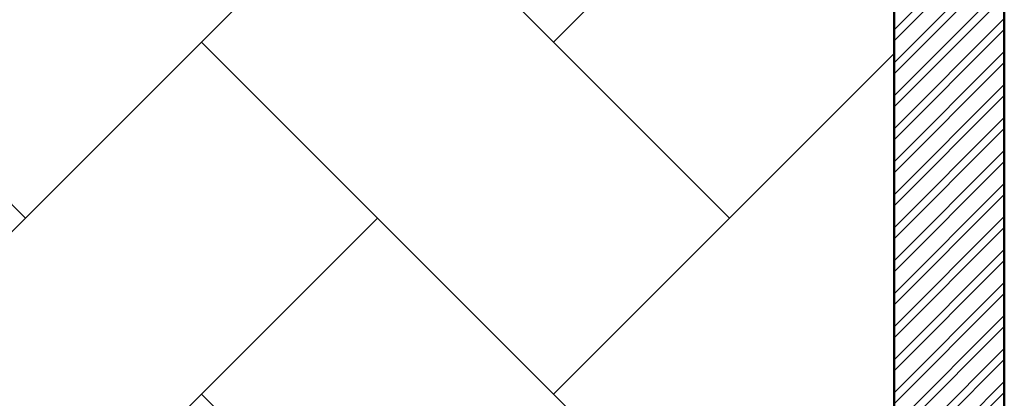
# Model space of a CAD drawing. Units: inches. Extents: x 3590 to 5167, y 65 to 1917.
# Tile 62 of 100: x 5000 to 5080, y 1609 to 1640. Entities that reach past the tile are written whole.
import ezdxf

# ---------------------------------------------------------------- set-up
doc = ezdxf.new("R2010")
doc.units = ezdxf.units.IN
for name, color, linetype, lineweight in [('A-FLOR-PATT', 8, 'Continuous', 13), ('A-WALL', 7, 'Continuous', 50), ('A-WALL-PATT', 251, 'Continuous', 13)]:
    doc.layers.add(name, color=color, linetype=linetype, lineweight=lineweight)

msp = doc.modelspace()

# ---------------------------------------------------------------- hatches: boundary and pattern name
at = {"layer": 'A-FLOR-PATT', "transparency": 33554687}
h = msp.add_hatch(dxfattribs=at)
h.set_pattern_fill('AR-HBONE', color=256, scale=0.2)
h.set_pattern_definition([(45, (-588.972, 0), (0, 28.73682), [60.96, -20.32]), (135, (-574.604, 14.368), (3e-15, 28.73682), [60.96, -20.32])])
h.paths.add_polyline_path([(5071.274, 1796.999), (4933.274, 1796.999), (4933.274, 1753.999), (4962.774, 1753.999, -0.414214), (4928.774, 1719.999), (4933.274, 1718.999), (4933.274, 1334.999), (5071.274, 1334.999)])
h.paths.add_polyline_path([(4951.78, 1521.077), (4951.715, 1521.04), (4951.563, 1520.895)], flags=16)
h.paths.add_polyline_path([(4952.267, 1521.376), (4952.198, 1521.371), (4952.198, 1521.356)], flags=0)
h.paths.add_polyline_path([(4967.051, 1529.728), (4965.231, 1528.694), (4963.411, 1527.714), (4961.756, 1526.851), (4963.589, 1527.449), (4964.036, 1527.478), (4962.975, 1527.249), (4961.76, 1526.852), (4959.792, 1525.834), (4958.005, 1524.895), (4956.24, 1523.93), (4954.504, 1522.919), (4954.129, 1522.682), (4953.361, 1521.997), (4953.366, 1521.998), (4953.605, 1522.064), (4955.106, 1522.761), (4956.921, 1523.434), (4958.678, 1523.915), (4960.358, 1524.2), (4961.945, 1524.286), (4964.171, 1524.108), (4965.958, 1523.309), (4963.863, 1522.976), (4965.187, 1522.499), (4963.366, 1522.497), (4961.545, 1522.487), (4959.764, 1522.461), (4958.304, 1522.419), (4957.974, 1522.388), (4956.307, 1522.232), (4954.718, 1522.071), (4953.251, 1521.899), (4953.525, 1521.623), (4954.331, 1521.379), (4956.243, 1521.23), (4958.039, 1520.93), (4959.684, 1520.483), (4961.16, 1519.896), (4963.107, 1518.8), (4964.393, 1517.325), (4962.973, 1517.726), (4964.558, 1516.661), (4965.407, 1515.708), (4963.507, 1516.322), (4961.68, 1517.005), (4959.935, 1517.745), (4958.282, 1518.528), (4956.732, 1519.343), (4955.295, 1520.175), (4954.672, 1520.572), (4954.513, 1520.627), (4955.658, 1519.318), (4956.703, 1517.982), (4957.644, 1516.647), (4958.485, 1515.334), (4959.55, 1513.524), (4960.438, 1511.769), (4958.841, 1513.62), (4957.452, 1515.325), (4955.819, 1517.459), (4956.665, 1515.448), (4957.111, 1513.923), (4957.447, 1511.714), (4957.076, 1509.793), (4956.538, 1511.11), (4955.992, 1512.569), (4955.444, 1514.125), (4954.898, 1515.735), (4954.357, 1517.356), (4953.824, 1518.943), (4953.305, 1520.452), (4953.065, 1521.116), (4952.971, 1521.146), (4952.949, 1521.086), (4952.73, 1520.199), (4953.37, 1518.024), (4953.757, 1516.373), (4954.051, 1514.765), (4954.264, 1513.221), (4954.471, 1511.131), (4954.497, 1510.402), (4954.409, 1511.76), (4954.264, 1513.221), (4954.051, 1514.765), (4953.757, 1516.373), (4953.37, 1518.024), (4952.877, 1519.698), (4952.716, 1520.141), (4952.533, 1519.059), (4952.374, 1517.789), (4952.219, 1516.312), (4952.046, 1514.6), (4951.833, 1512.626), (4951.557, 1510.363), (4951.203, 1512.168), (4950.852, 1514.339), (4950.985, 1516.376), (4951.66, 1518.286), (4952.593, 1520.481), (4952.357, 1521.13), (4951.855, 1520.328), (4950.839, 1518.908), (4949.777, 1517.587), (4948.916, 1516.617), (4948.111, 1515.256), (4947.089, 1513.554), (4945.889, 1511.615), (4946.326, 1513.402), (4946.562, 1514.249), (4945.528, 1513.327), (4944.581, 1512.531), (4946.018, 1514.508), (4947.204, 1516.048), (4947.893, 1517.313), (4949.307, 1518.764), (4950.414, 1519.767), (4950.451, 1519.806), (4952.267, 1521.376), (4951.645, 1521.493), (4950.404, 1521.18), (4948.044, 1520.359), (4946.119, 1519.452), (4944.572, 1518.475), (4943.35, 1517.443), (4941.997, 1515.92), (4941.661, 1515.275), (4942.813, 1516.99), (4944.572, 1518.475), (4946.119, 1519.452), (4948.044, 1520.359), (4950.404, 1521.18), (4951.645, 1521.493), (4949.647, 1521.868), (4948.6, 1521.756), (4947.126, 1521.57), (4945.42, 1521.348), (4943.45, 1521.105), (4941.183, 1520.856), (4942.86, 1521.613), (4943.873, 1522.03), (4942.952, 1521.909), (4941.41, 1521.485), (4939.543, 1520.67), (4938.968, 1520.226), (4940.733, 1521.299), (4942.952, 1521.909), (4943.702, 1522.008), (4945.894, 1522.7), (4947.565, 1522.714), (4948.921, 1522.566), (4951.131, 1522.183), (4950.971, 1522.297), (4948.129, 1523.006), (4946.035, 1523.707), (4944.232, 1524.521), (4942.707, 1525.461), (4941.444, 1526.537), (4940.43, 1527.761), (4939.649, 1529.143), (4941.421, 1528.122), (4943.147, 1527.132), (4944.841, 1526.175), (4946.514, 1525.25), (4948.179, 1524.359), (4948.365, 1524.263), (4946.475, 1526.045), (4945.181, 1527.54), (4944.19, 1529.033), (4943.496, 1530.54), (4943.278, 1531.36), (4942.498, 1531.919), (4943.114, 1531.762), (4942.959, 1533.659), (4944.14, 1531.989), (4944.612, 1531.323), (4946.202, 1530.463), (4947.486, 1529.509), (4948.79, 1528.226), (4950.368, 1526.237), (4949.485, 1528.155), (4948.851, 1530.123), (4948.491, 1532.041), (4948.381, 1533.918), (4948.501, 1535.76), (4948.827, 1537.573), (4949.418, 1535.565), (4949.957, 1533.569), (4950.464, 1531.586), (4950.961, 1529.617), (4951.391, 1527.954), (4951.724, 1530.687), (4952.201, 1532.58), (4952.889, 1534.33), (4953.77, 1535.951), (4954.827, 1537.46), (4954.521, 1535.39), (4954.273, 1533.937), (4955.58, 1535.663), (4956.748, 1536.739), (4956.159, 1534.78), (4955.589, 1532.873), (4955.043, 1531.006), (4954.525, 1529.166), (4954.038, 1527.341), (4953.638, 1525.733), (4953.611, 1525.586), (4953.398, 1524.166), (4953.382, 1524.009), (4954.07, 1525.476), (4954.912, 1527.022), (4956.136, 1528.894), (4957.847, 1530.577), (4959.376, 1531.54), (4958.256, 1530.104), (4957.143, 1528.663), (4956.066, 1527.243), (4955.056, 1525.871), (4954.141, 1524.571), (4953.352, 1523.372), (4953.311, 1523.303), (4953.273, 1522.925), (4953.261, 1522.382), (4954.103, 1523.373), (4954.63, 1524.284), (4955.961, 1526.358), (4957.23, 1528.13), (4958.421, 1529.609), (4960.037, 1531.368), (4961.374, 1532.375), (4962.101, 1532.77), (4961.07, 1531.061), (4959.987, 1529.438), (4958.869, 1527.908), (4958.15, 1527.007), (4959.803, 1528.003), (4961.589, 1528.793), (4963.391, 1529.328), (4965.211, 1529.632)], flags=16)
h.paths.add_polyline_path([(4962.944, 1523.182), (4961.107, 1523.422), (4960.392, 1523.362), (4962.35, 1523.331)], flags=0)
h.paths.add_polyline_path([(5049.541, 1584.551), (5049.476, 1584.515), (5049.325, 1584.37)], flags=16)
h.paths.add_polyline_path([(5050.028, 1584.851), (5049.959, 1584.845), (5049.959, 1584.83)], flags=0)
h.paths.add_polyline_path([(5042.333, 1581.949), (5043.88, 1582.926), (5045.806, 1583.833), (5048.165, 1584.654), (5049.406, 1584.967), (5047.408, 1585.342), (5046.361, 1585.231), (5044.888, 1585.044), (5043.181, 1584.822), (5041.211, 1584.579), (5038.944, 1584.33), (5040.622, 1585.087), (5041.634, 1585.504), (5040.713, 1585.383), (5039.171, 1584.959), (5037.304, 1584.144), (5036.729, 1583.7), (5038.494, 1584.773), (5040.713, 1585.383), (5041.463, 1585.482), (5043.655, 1586.174), (5045.326, 1586.188), (5046.682, 1586.04), (5048.893, 1585.657), (5048.732, 1585.771), (5045.891, 1586.48), (5043.796, 1587.181), (5041.994, 1587.996), (5040.468, 1588.935), (5039.205, 1590.011), (5038.191, 1591.235), (5037.41, 1592.617), (5039.182, 1591.596), (5040.909, 1590.607), (5042.602, 1589.649), (5044.275, 1588.724), (5045.94, 1587.833), (5046.126, 1587.738), (5044.237, 1589.519), (5042.942, 1591.015), (5041.952, 1592.508), (5041.257, 1594.014), (5041.039, 1594.834), (5040.26, 1595.393), (5040.875, 1595.237), (5040.721, 1597.133), (5041.901, 1595.463), (5042.373, 1594.798), (5043.963, 1593.938), (5045.247, 1592.983), (5046.552, 1591.701), (5048.129, 1589.712), (5047.247, 1591.63), (5046.613, 1593.597), (5046.252, 1595.515), (5046.142, 1597.392), (5046.262, 1599.234), (5046.588, 1601.047), (5047.179, 1599.039), (5047.718, 1597.043), (5048.225, 1595.06), (5048.722, 1593.091), (5049.152, 1591.429), (5049.485, 1594.161), (5049.962, 1596.054), (5050.65, 1597.804), (5051.532, 1599.425), (5052.589, 1600.934), (5052.283, 1598.864), (5052.034, 1597.411), (5053.341, 1599.137), (5054.509, 1600.213), (5053.92, 1598.254), (5053.35, 1596.348), (5052.805, 1594.48), (5052.286, 1592.64), (5051.799, 1590.815), (5051.4, 1589.207), (5051.373, 1589.06), (5051.159, 1587.64), (5051.143, 1587.483), (5051.831, 1588.95), (5052.673, 1590.496), (5053.898, 1592.368), (5055.608, 1594.051), (5057.137, 1595.014), (5056.017, 1593.578), (5054.904, 1592.137), (5053.828, 1590.717), (5052.817, 1589.345), (5051.902, 1588.046), (5051.113, 1586.846), (5051.072, 1586.777), (5051.034, 1586.399), (5051.022, 1585.856), (5051.864, 1586.847), (5052.391, 1587.758), (5053.723, 1589.832), (5054.991, 1591.604), (5056.182, 1593.083), (5057.798, 1594.842), (5059.135, 1595.849), (5059.863, 1596.244), (5058.831, 1594.535), (5057.749, 1592.912), (5056.63, 1591.382), (5055.912, 1590.482), (5057.564, 1591.477), (5059.35, 1592.267), (5061.152, 1592.802), (5062.972, 1593.106), (5064.812, 1593.203), (5062.992, 1592.169), (5061.172, 1591.188), (5059.518, 1590.325), (5061.35, 1590.924), (5061.797, 1590.952), (5060.737, 1590.723), (5059.521, 1590.326), (5057.553, 1589.308), (5055.766, 1588.369), (5054.002, 1587.404), (5052.265, 1586.393), (5051.891, 1586.156), (5051.122, 1585.471), (5051.127, 1585.472), (5051.366, 1585.538), (5052.867, 1586.235), (5054.682, 1586.908), (5056.439, 1587.389), (5058.12, 1587.675), (5059.706, 1587.76), (5061.933, 1587.583), (5063.719, 1586.783), (5061.624, 1586.45), (5062.949, 1585.973), (5061.127, 1585.971), (5059.307, 1585.961), (5057.525, 1585.935), (5056.065, 1585.893), (5055.735, 1585.862), (5054.068, 1585.707), (5052.479, 1585.546), (5051.012, 1585.373), (5051.286, 1585.097), (5052.092, 1584.853), (5054.004, 1584.704), (5055.8, 1584.404), (5057.446, 1583.958), (5058.921, 1583.37), (5060.868, 1582.274), (5062.154, 1580.799), (5060.734, 1581.2), (5062.32, 1580.135), (5063.168, 1579.182), (5061.269, 1579.796), (5059.441, 1580.479), (5057.696, 1581.219), (5056.043, 1582.003), (5054.493, 1582.817), (5053.057, 1583.649), (5052.433, 1584.047), (5052.274, 1584.101), (5053.42, 1582.793), (5054.464, 1581.457), (5055.405, 1580.121), (5056.247, 1578.809), (5057.311, 1576.998), (5058.199, 1575.244), (5056.602, 1577.094), (5055.213, 1578.799), (5053.58, 1580.933), (5054.427, 1578.922), (5054.872, 1577.397), (5055.208, 1575.189), (5054.838, 1573.267), (5054.299, 1574.584), (5053.754, 1576.043), (5053.206, 1577.599), (5052.659, 1579.209), (5052.118, 1580.83), (5051.585, 1582.417), (5051.066, 1583.927), (5050.826, 1584.59), (5050.733, 1584.62), (5050.711, 1584.561), (5050.491, 1583.673), (5051.131, 1581.498), (5051.518, 1579.847), (5051.813, 1578.24), (5052.026, 1576.695), (5052.233, 1574.605), (5052.258, 1573.876), (5052.17, 1575.234), (5052.026, 1576.695), (5051.813, 1578.24), (5051.518, 1579.847), (5051.131, 1581.498), (5050.638, 1583.172), (5050.477, 1583.615), (5050.294, 1582.533), (5050.136, 1581.263), (5049.981, 1579.786), (5049.807, 1578.074), (5049.594, 1576.1), (5049.318, 1573.837), (5048.965, 1575.642), (5048.613, 1577.813), (5048.747, 1579.85), (5049.421, 1581.76), (5050.354, 1583.955), (5050.118, 1584.604), (5049.616, 1583.802), (5048.6, 1582.382), (5047.538, 1581.061), (5046.677, 1580.091), (5045.872, 1578.73), (5044.85, 1577.028), (5043.651, 1575.089), (5044.087, 1576.877), (5044.324, 1577.723), (5043.289, 1576.801), (5042.342, 1576.005), (5043.779, 1577.982), (5044.966, 1579.522), (5045.655, 1580.787), (5047.068, 1582.239), (5048.175, 1583.241), (5048.213, 1583.28), (5050.028, 1584.851), (5049.406, 1584.967), (5048.165, 1584.654), (5045.806, 1583.833), (5043.88, 1582.926), (5042.333, 1581.949), (5041.111, 1580.917), (5039.758, 1579.394), (5039.423, 1578.749), (5040.575, 1580.464)], flags=16)
h.paths.add_polyline_path([(4954.799, 1533.12), (4954.262, 1532.079), (4953.831, 1530.935), (4953.505, 1529.636), (4953.283, 1528.133), (4953.167, 1526.376), (4953.156, 1524.315), (4953.277, 1521.236), (4952.802, 1521.842), (4951.557, 1521.998), (4950.976, 1521.961), (4952.661, 1521.941), (4952.802, 1521.842), (4953.152, 1523.593), (4953.167, 1526.376), (4953.283, 1528.133), (4953.609, 1530.346), (4954.456, 1532.592)], flags=0)
h.paths.add_polyline_path([(5050.563, 1585.316), (5049.318, 1585.472), (5048.737, 1585.435), (5050.422, 1585.415), (5050.563, 1585.316), (5050.914, 1587.067), (5050.928, 1589.851), (5051.045, 1591.607), (5051.371, 1593.82), (5052.217, 1596.066), (5052.56, 1596.594), (5052.024, 1595.554), (5051.592, 1594.409), (5051.266, 1593.11), (5051.045, 1591.607), (5050.928, 1589.851), (5050.918, 1587.789), (5051.038, 1584.71)], flags=0)
h.paths.add_polyline_path([(5058.153, 1586.836), (5060.111, 1586.805), (5060.705, 1586.656), (5058.868, 1586.896)], flags=0)
h.paths.add_polyline_path([(5049.541, 1430.936), (5049.476, 1430.9), (5049.325, 1430.755)], flags=16)
h.paths.add_polyline_path([(5050.028, 1431.236), (5049.959, 1431.231), (5049.959, 1431.215)], flags=0)
h.paths.add_polyline_path([(5046.588, 1447.432), (5047.179, 1445.425), (5047.718, 1443.429), (5048.225, 1441.446), (5048.722, 1439.476), (5049.152, 1437.814), (5049.485, 1440.546), (5049.962, 1442.439), (5050.65, 1444.189), (5051.532, 1445.811), (5052.589, 1447.319), (5052.283, 1445.249), (5052.034, 1443.796), (5053.341, 1445.522), (5054.509, 1446.598), (5053.92, 1444.64), (5053.35, 1442.733), (5052.805, 1440.865), (5052.286, 1439.025), (5051.799, 1437.201), (5051.4, 1435.592), (5051.373, 1435.445), (5051.159, 1434.025), (5051.143, 1433.868), (5051.831, 1435.335), (5052.673, 1436.881), (5053.898, 1438.753), (5055.608, 1440.436), (5057.137, 1441.4), (5056.017, 1439.963), (5054.904, 1438.522), (5053.828, 1437.102), (5052.817, 1435.73), (5051.902, 1434.431), (5051.113, 1433.231), (5051.072, 1433.162), (5051.034, 1432.784), (5051.022, 1432.242), (5051.864, 1433.232), (5052.391, 1434.143), (5053.723, 1436.217), (5054.991, 1437.989), (5056.182, 1439.468), (5057.798, 1441.227), (5059.135, 1442.235), (5059.863, 1442.629), (5058.831, 1440.921), (5057.749, 1439.298), (5056.63, 1437.767), (5055.912, 1436.867), (5057.564, 1437.863), (5059.35, 1438.652), (5061.152, 1439.187), (5062.972, 1439.491), (5064.812, 1439.588), (5062.992, 1438.554), (5061.172, 1437.573), (5059.518, 1436.71), (5061.35, 1437.309), (5061.797, 1437.337), (5060.737, 1437.108), (5059.521, 1436.711), (5057.553, 1435.693), (5055.766, 1434.754), (5054.002, 1433.789), (5052.265, 1432.778), (5051.891, 1432.541), (5051.122, 1431.856), (5051.127, 1431.857), (5051.366, 1431.923), (5052.867, 1432.62), (5054.682, 1433.293), (5056.439, 1433.775), (5058.12, 1434.06), (5059.706, 1434.145), (5061.933, 1433.968), (5063.719, 1433.168), (5061.624, 1432.835), (5062.949, 1432.358), (5061.127, 1432.357), (5059.307, 1432.346), (5057.525, 1432.32), (5056.065, 1432.278), (5055.735, 1432.248), (5054.068, 1432.092), (5052.479, 1431.931), (5051.012, 1431.759), (5051.286, 1431.482), (5052.092, 1431.238), (5054.004, 1431.089), (5055.8, 1430.789), (5057.446, 1430.343), (5058.921, 1429.755), (5060.868, 1428.66), (5062.154, 1427.185), (5060.734, 1427.585), (5062.32, 1426.52), (5063.168, 1425.567), (5061.269, 1426.181), (5059.441, 1426.865), (5057.696, 1427.604), (5056.043, 1428.388), (5054.493, 1429.202), (5053.057, 1430.034), (5052.433, 1430.432), (5052.274, 1430.487), (5053.42, 1429.178), (5054.464, 1427.842), (5055.405, 1426.506), (5056.247, 1425.194), (5057.311, 1423.383), (5058.199, 1421.629), (5056.602, 1423.479), (5055.213, 1425.184), (5053.58, 1427.318), (5054.427, 1425.307), (5054.872, 1423.782), (5055.208, 1421.574), (5054.838, 1419.652), (5054.299, 1420.97), (5053.754, 1422.428), (5053.206, 1423.984), (5052.659, 1425.595), (5052.118, 1427.215), (5051.585, 1428.802), (5051.066, 1430.312), (5050.826, 1430.975), (5050.733, 1431.005), (5050.711, 1430.946), (5050.491, 1430.058), (5051.131, 1427.883), (5051.518, 1426.232), (5051.813, 1424.625), (5052.026, 1423.081), (5052.233, 1420.991), (5052.258, 1420.261), (5052.17, 1421.619), (5052.026, 1423.081), (5051.813, 1424.625), (5051.518, 1426.232), (5051.131, 1427.883), (5050.638, 1429.558), (5050.477, 1430.001), (5050.294, 1428.918), (5050.136, 1427.648), (5049.981, 1426.171), (5049.807, 1424.459), (5049.594, 1422.485), (5049.318, 1420.222), (5048.965, 1422.028), (5048.613, 1424.199), (5048.747, 1426.235), (5049.421, 1428.146), (5050.354, 1430.34), (5050.118, 1430.989), (5049.616, 1430.187), (5048.6, 1428.768), (5047.538, 1427.446), (5046.677, 1426.477), (5045.872, 1425.116), (5044.85, 1423.413), (5043.651, 1421.474), (5044.087, 1423.262), (5044.324, 1424.109), (5043.289, 1423.186), (5042.342, 1422.391), (5043.779, 1424.368), (5044.966, 1425.907), (5045.655, 1427.173), (5047.068, 1428.624), (5048.175, 1429.627), (5048.213, 1429.666), (5050.028, 1431.236), (5049.406, 1431.353), (5048.165, 1431.039), (5045.806, 1430.218), (5043.88, 1429.311), (5042.333, 1428.334), (5041.111, 1427.302), (5039.758, 1425.779), (5039.423, 1425.134), (5040.575, 1426.849), (5042.333, 1428.334), (5043.88, 1429.311), (5045.806, 1430.218), (5048.165, 1431.039), (5049.406, 1431.353), (5047.408, 1431.727), (5046.361, 1431.616), (5044.888, 1431.429), (5043.181, 1431.207), (5041.211, 1430.964), (5038.944, 1430.715), (5040.622, 1431.472), (5041.634, 1431.89), (5040.713, 1431.769), (5039.171, 1431.345), (5037.304, 1430.53), (5036.729, 1430.085), (5038.494, 1431.158), (5040.713, 1431.769), (5041.463, 1431.867), (5043.655, 1432.559), (5045.326, 1432.573), (5046.682, 1432.425), (5048.893, 1432.042), (5048.732, 1432.156), (5045.891, 1432.865), (5043.796, 1433.566), (5041.994, 1434.381), (5040.468, 1435.321), (5039.205, 1436.396), (5038.191, 1437.62), (5037.41, 1439.002), (5039.182, 1437.982), (5040.909, 1436.992), (5042.602, 1436.034), (5044.275, 1435.109), (5045.94, 1434.218), (5046.126, 1434.123), (5044.237, 1435.904), (5042.942, 1437.4), (5041.952, 1438.893), (5041.257, 1440.399), (5041.039, 1441.219), (5040.26, 1441.778), (5040.875, 1441.622), (5040.721, 1443.518), (5041.901, 1441.848), (5042.373, 1441.183), (5043.963, 1440.323), (5045.247, 1439.369), (5046.552, 1438.086), (5048.129, 1436.097), (5047.247, 1438.015), (5046.613, 1439.982), (5046.252, 1441.901), (5046.142, 1443.778), (5046.262, 1445.619)], flags=16)
h.paths.add_polyline_path([(5052.382, 1444.255), (5051.623, 1442.78), (5052.024, 1441.939), (5052.56, 1442.98)], flags=0)
h.paths.add_polyline_path([(5050.563, 1431.701), (5049.318, 1431.857), (5048.737, 1431.821), (5050.422, 1431.8)], flags=0)
h.paths.add_polyline_path([(5058.153, 1433.221), (5060.111, 1433.19), (5060.705, 1433.041), (5058.868, 1433.281)], flags=0)
h.paths.add_polyline_path([(5049.541, 1352.285), (5049.476, 1352.249), (5049.325, 1352.104)], flags=16)
h.paths.add_polyline_path([(5050.028, 1352.585), (5049.959, 1352.58), (5049.959, 1352.564)], flags=0)
h.paths.add_polyline_path([(5046.588, 1368.781), (5047.179, 1366.774), (5047.718, 1364.778), (5048.225, 1362.795), (5048.722, 1360.825), (5049.152, 1359.163), (5049.485, 1361.896), (5049.962, 1363.789), (5050.65, 1365.538), (5051.532, 1367.16), (5052.589, 1368.669), (5052.283, 1366.598), (5052.034, 1365.145), (5053.341, 1366.871), (5054.509, 1367.947), (5053.92, 1365.989), (5053.35, 1364.082), (5052.805, 1362.214), (5052.286, 1360.374), (5051.799, 1358.55), (5051.4, 1356.942), (5051.373, 1356.794), (5051.159, 1355.374), (5051.143, 1355.218), (5051.831, 1356.684), (5052.673, 1358.23), (5053.898, 1360.102), (5055.608, 1361.786), (5057.137, 1362.749), (5056.017, 1361.313), (5054.904, 1359.872), (5053.828, 1358.452), (5052.817, 1357.079), (5051.902, 1355.78), (5051.113, 1354.581), (5051.072, 1354.512), (5051.034, 1354.133), (5051.022, 1353.591), (5051.864, 1354.581), (5052.391, 1355.492), (5053.723, 1357.566), (5054.991, 1359.338), (5056.182, 1360.817), (5057.798, 1362.577), (5059.135, 1363.584), (5059.863, 1363.979), (5058.831, 1362.27), (5057.749, 1360.647), (5056.63, 1359.117), (5055.912, 1358.216), (5057.564, 1359.212), (5059.35, 1360.001), (5061.152, 1360.536), (5062.972, 1360.841), (5064.812, 1360.937), (5062.992, 1359.903), (5061.172, 1358.923), (5059.518, 1358.059), (5061.35, 1358.658), (5061.797, 1358.687), (5060.737, 1358.458), (5059.521, 1358.061), (5057.553, 1357.043), (5055.766, 1356.103), (5054.002, 1355.138), (5052.265, 1354.127), (5051.891, 1353.89), (5051.122, 1353.206), (5051.127, 1353.206), (5051.366, 1353.272), (5052.867, 1353.969), (5054.682, 1354.643), (5056.439, 1355.124), (5058.12, 1355.409), (5059.706, 1355.495), (5061.933, 1355.317), (5063.719, 1354.518), (5061.624, 1354.184), (5062.949, 1353.708), (5061.127, 1353.706), (5059.307, 1353.695), (5057.525, 1353.669), (5056.065, 1353.627), (5055.735, 1353.597), (5054.068, 1353.441), (5052.479, 1353.28), (5051.012, 1353.108), (5051.286, 1352.831), (5052.092, 1352.587), (5054.004, 1352.439), (5055.8, 1352.138), (5057.446, 1351.692), (5058.921, 1351.104), (5060.868, 1350.009), (5062.154, 1348.534), (5060.734, 1348.935), (5062.32, 1347.869), (5063.168, 1346.916), (5061.269, 1347.53), (5059.441, 1348.214), (5057.696, 1348.954), (5056.043, 1349.737), (5054.493, 1350.551), (5053.057, 1351.383), (5052.433, 1351.781), (5052.274, 1351.836), (5053.42, 1350.527), (5054.464, 1349.191), (5055.405, 1347.855), (5056.247, 1346.543), (5057.311, 1344.733), (5058.199, 1342.978), (5056.602, 1344.828), (5055.213, 1346.534), (5053.58, 1348.667), (5054.427, 1346.656), (5054.872, 1345.132), (5055.208, 1342.923), (5054.838, 1341.002), (5054.299, 1342.319), (5053.754, 1343.778), (5053.206, 1345.334), (5052.659, 1346.944), (5052.118, 1348.564), (5051.585, 1350.151), (5051.066, 1351.661), (5050.826, 1352.324), (5050.733, 1352.355), (5050.711, 1352.295), (5050.491, 1351.408), (5051.131, 1349.232), (5051.518, 1347.581), (5051.813, 1345.974), (5052.026, 1344.43), (5052.233, 1342.34), (5052.258, 1341.61), (5052.17, 1342.969), (5052.026, 1344.43), (5051.813, 1345.974), (5051.518, 1347.581), (5051.131, 1349.232), (5050.638, 1350.907), (5050.477, 1351.35), (5050.294, 1350.267), (5050.136, 1348.997), (5049.981, 1347.52), (5049.807, 1345.809), (5049.594, 1343.835), (5049.318, 1341.571), (5048.965, 1343.377), (5048.613, 1345.548), (5048.747, 1347.585), (5049.421, 1349.495), (5050.354, 1351.689), (5050.118, 1352.339), (5049.616, 1351.536), (5048.6, 1350.117), (5047.538, 1348.795), (5046.677, 1347.826), (5045.872, 1346.465), (5044.85, 1344.763), (5043.651, 1342.824), (5044.087, 1344.611), (5044.324, 1345.458), (5043.289, 1344.535), (5042.342, 1343.74), (5043.779, 1345.717), (5044.966, 1347.256), (5045.655, 1348.522), (5047.068, 1349.973), (5048.175, 1350.976), (5048.213, 1351.015), (5050.028, 1352.585), (5049.406, 1352.702), (5048.165, 1352.388), (5045.806, 1351.567), (5043.88, 1350.661), (5042.333, 1349.683), (5041.111, 1348.651), (5039.758, 1347.128), (5039.423, 1346.483), (5040.575, 1348.198), (5042.333, 1349.683), (5043.88, 1350.661), (5045.806, 1351.567), (5048.165, 1352.388), (5049.406, 1352.702), (5047.408, 1353.076), (5046.361, 1352.965), (5044.888, 1352.779), (5043.181, 1352.556), (5041.211, 1352.313), (5038.944, 1352.065), (5040.622, 1352.821), (5041.634, 1353.239), (5040.713, 1353.118), (5039.171, 1352.694), (5037.304, 1351.879), (5036.729, 1351.434), (5038.494, 1352.508), (5040.713, 1353.118), (5041.463, 1353.216), (5043.655, 1353.909), (5045.326, 1353.923), (5046.682, 1353.774), (5048.893, 1353.391), (5048.732, 1353.506), (5045.891, 1354.214), (5043.796, 1354.915), (5041.994, 1355.73), (5040.468, 1356.67), (5039.205, 1357.746), (5038.191, 1358.969), (5037.41, 1360.352), (5039.182, 1359.331), (5040.909, 1358.341), (5042.602, 1357.383), (5044.275, 1356.458), (5045.94, 1355.567), (5046.126, 1355.472), (5044.237, 1357.253), (5042.942, 1358.749), (5041.952, 1360.242), (5041.257, 1361.748), (5041.039, 1362.568), (5040.26, 1363.128), (5040.875, 1362.971), (5040.721, 1364.867), (5041.901, 1363.197), (5042.373, 1362.532), (5043.963, 1361.672), (5045.247, 1360.718), (5046.552, 1359.435), (5048.129, 1357.446), (5047.247, 1359.364), (5046.613, 1361.331), (5046.252, 1363.25), (5046.142, 1365.127), (5046.262, 1366.969)], flags=16)
h.paths.add_polyline_path([(5052.382, 1365.604), (5051.623, 1364.129), (5052.024, 1363.288), (5052.56, 1364.329)], flags=0)
h.paths.add_polyline_path([(4951.78, 1698.041), (4951.715, 1698.005), (4951.563, 1697.859)], flags=16)
h.paths.add_polyline_path([(4952.267, 1698.341), (4952.198, 1698.335), (4952.198, 1698.32)], flags=0)
h.paths.add_polyline_path([(4957.076, 1686.757), (4956.538, 1688.074), (4955.992, 1689.533), (4955.444, 1691.089), (4954.898, 1692.699), (4954.357, 1694.32), (4953.824, 1695.907), (4953.305, 1697.417), (4953.065, 1698.08), (4952.971, 1698.11), (4952.949, 1698.051), (4952.73, 1697.163), (4953.37, 1694.988), (4953.757, 1693.337), (4954.051, 1691.729), (4954.264, 1690.185), (4954.471, 1688.095), (4954.497, 1687.366), (4954.409, 1688.724), (4954.264, 1690.185), (4954.051, 1691.729), (4953.757, 1693.337), (4953.37, 1694.988), (4952.877, 1696.662), (4952.716, 1697.105), (4952.533, 1696.023), (4952.374, 1694.753), (4952.219, 1693.276), (4952.046, 1691.564), (4951.833, 1689.59), (4951.557, 1687.327), (4951.203, 1689.132), (4950.852, 1691.303), (4950.985, 1693.34), (4951.66, 1695.25), (4952.593, 1697.445), (4952.357, 1698.094), (4951.855, 1697.292), (4950.839, 1695.872), (4949.777, 1694.551), (4948.916, 1693.581), (4948.111, 1692.22), (4947.089, 1690.518), (4945.889, 1688.579), (4946.326, 1690.366), (4946.562, 1691.213), (4945.528, 1690.291), (4944.581, 1689.495), (4946.018, 1691.472), (4947.204, 1693.012), (4947.893, 1694.277), (4949.307, 1695.729), (4950.414, 1696.731), (4950.451, 1696.77), (4952.267, 1698.341), (4951.645, 1698.457), (4950.404, 1698.144), (4948.044, 1697.323), (4946.119, 1696.416), (4944.572, 1695.439), (4943.35, 1694.407), (4941.997, 1692.884), (4941.661, 1692.239), (4942.813, 1693.954), (4944.572, 1695.439), (4946.119, 1696.416), (4948.044, 1697.323), (4950.404, 1698.144), (4951.645, 1698.457), (4949.647, 1698.832), (4948.6, 1698.72), (4947.126, 1698.534), (4945.42, 1698.312), (4943.45, 1698.069), (4941.183, 1697.82), (4942.86, 1698.577), (4943.873, 1698.994), (4942.952, 1698.873), (4941.41, 1698.449), (4939.543, 1697.634), (4938.968, 1697.19), (4940.733, 1698.263), (4942.952, 1698.873), (4943.702, 1698.972), (4945.894, 1699.664), (4947.565, 1699.678), (4948.921, 1699.53), (4951.131, 1699.147), (4950.971, 1699.261), (4948.129, 1699.97), (4946.035, 1700.671), (4944.232, 1701.486), (4942.707, 1702.425), (4941.444, 1703.501), (4940.43, 1704.725), (4939.649, 1706.107), (4941.421, 1705.086), (4943.147, 1704.097), (4944.841, 1703.139), (4946.514, 1702.214), (4948.179, 1701.323), (4948.365, 1701.227), (4946.475, 1703.009), (4945.181, 1704.505), (4944.19, 1705.997), (4943.496, 1707.504), (4943.278, 1708.324), (4942.498, 1708.883), (4943.114, 1708.727), (4942.959, 1710.623), (4944.14, 1708.953), (4944.612, 1708.287), (4946.202, 1707.428), (4947.486, 1706.473), (4948.79, 1705.191), (4950.368, 1703.202), (4949.485, 1705.12), (4948.851, 1707.087), (4948.491, 1709.005), (4948.381, 1710.882), (4948.501, 1712.724), (4948.827, 1714.537), (4949.418, 1712.529), (4949.957, 1710.533), (4950.464, 1708.55), (4950.961, 1706.581), (4951.391, 1704.919), (4951.724, 1707.651), (4952.201, 1709.544), (4952.889, 1711.294), (4953.77, 1712.915), (4954.827, 1714.424), (4954.521, 1712.354), (4954.273, 1710.901), (4955.58, 1712.627), (4956.748, 1713.703), (4956.159, 1711.744), (4955.589, 1709.837), (4955.043, 1707.97), (4954.525, 1706.13), (4954.038, 1704.305), (4953.638, 1702.697), (4953.611, 1702.55), (4953.398, 1701.13), (4953.382, 1700.973), (4954.07, 1702.44), (4954.912, 1703.986), (4956.136, 1705.858), (4957.847, 1707.541), (4959.376, 1708.504), (4958.256, 1707.068), (4957.143, 1705.627), (4956.066, 1704.207), (4955.056, 1702.835), (4954.141, 1701.536), (4953.352, 1700.336), (4953.311, 1700.267), (4953.273, 1699.889), (4953.261, 1699.346), (4954.103, 1700.337), (4954.63, 1701.248), (4955.961, 1703.322), (4957.23, 1705.094), (4958.421, 1706.573), (4960.037, 1708.332), (4961.374, 1709.339), (4962.101, 1709.734), (4961.07, 1708.025), (4959.987, 1706.402), (4958.869, 1704.872), (4958.15, 1703.972), (4959.803, 1704.967), (4961.589, 1705.757), (4963.391, 1706.292), (4965.211, 1706.596), (4967.051, 1706.692), (4965.231, 1705.659), (4963.411, 1704.678), (4961.756, 1703.815), (4963.589, 1704.413), (4964.036, 1704.442), (4962.975, 1704.213), (4961.76, 1703.816), (4959.792, 1702.798), (4958.005, 1701.859), (4956.24, 1700.894), (4954.504, 1699.883), (4954.129, 1699.646), (4953.361, 1698.961), (4953.366, 1698.962), (4953.605, 1699.028), (4955.106, 1699.725), (4956.921, 1700.398), (4958.678, 1700.879), (4960.358, 1701.164), (4961.945, 1701.25), (4964.171, 1701.073), (4965.958, 1700.273), (4963.863, 1699.94), (4965.187, 1699.463), (4963.366, 1699.461), (4961.545, 1699.451), (4959.764, 1699.425), (4958.304, 1699.383), (4957.974, 1699.352), (4956.307, 1699.197), (4954.718, 1699.036), (4953.251, 1698.863), (4953.525, 1698.587), (4954.331, 1698.343), (4956.243, 1698.194), (4958.039, 1697.894), (4959.684, 1697.447), (4961.16, 1696.86), (4963.107, 1695.764), (4964.393, 1694.289), (4962.973, 1694.69), (4964.558, 1693.625), (4965.407, 1692.672), (4963.507, 1693.286), (4961.68, 1693.969), (4959.935, 1694.709), (4958.282, 1695.492), (4956.732, 1696.307), (4955.295, 1697.139), (4954.672, 1697.536), (4954.513, 1697.591), (4955.658, 1696.282), (4956.703, 1694.946), (4957.644, 1693.611), (4958.485, 1692.298), (4959.55, 1690.488), (4960.438, 1688.733), (4958.841, 1690.584), (4957.452, 1692.289), (4955.819, 1694.423), (4956.665, 1692.412), (4957.111, 1690.887), (4957.447, 1688.678)], flags=16)
h.paths.add_polyline_path([(5050.563, 1353.05), (5049.318, 1353.207), (5048.737, 1353.17), (5050.422, 1353.15)], flags=0)
h.paths.add_polyline_path([(4951.78, 1351.486), (4951.715, 1351.45), (4951.563, 1351.305)], flags=16)
h.paths.add_polyline_path([(4952.267, 1351.786), (4952.198, 1351.78), (4952.198, 1351.765)], flags=0)
h.paths.add_polyline_path([(4954.827, 1367.869), (4954.521, 1365.799), (4954.273, 1364.346), (4955.58, 1366.072), (4956.748, 1367.148), (4956.159, 1365.19), (4955.589, 1363.283), (4955.043, 1361.415), (4954.525, 1359.575), (4954.038, 1357.751), (4953.638, 1356.142), (4953.611, 1355.995), (4953.398, 1354.575), (4953.382, 1354.418), (4954.07, 1355.885), (4954.912, 1357.431), (4956.136, 1359.303), (4957.847, 1360.986), (4959.376, 1361.95), (4958.256, 1360.513), (4957.143, 1359.072), (4956.066, 1357.652), (4955.056, 1356.28), (4954.141, 1354.981), (4953.352, 1353.781), (4953.311, 1353.712), (4953.273, 1353.334), (4953.261, 1352.792), (4954.103, 1353.782), (4954.63, 1354.693), (4955.961, 1356.767), (4957.23, 1358.539), (4958.421, 1360.018), (4960.037, 1361.777), (4961.374, 1362.785), (4962.101, 1363.179), (4961.07, 1361.471), (4959.987, 1359.848), (4958.869, 1358.317), (4958.15, 1357.417), (4959.803, 1358.413), (4961.589, 1359.202), (4963.391, 1359.737), (4965.211, 1360.041), (4967.051, 1360.138), (4965.231, 1359.104), (4963.411, 1358.123), (4961.756, 1357.26), (4963.589, 1357.859), (4964.036, 1357.887), (4962.975, 1357.658), (4961.76, 1357.261), (4959.792, 1356.243), (4958.005, 1355.304), (4956.24, 1354.339), (4954.504, 1353.328), (4954.129, 1353.091), (4953.361, 1352.406), (4953.366, 1352.407), (4953.605, 1352.473), (4955.106, 1353.17), (4956.921, 1353.843), (4958.678, 1354.325), (4960.358, 1354.61), (4961.945, 1354.695), (4964.171, 1354.518), (4965.958, 1353.718), (4963.863, 1353.385), (4965.187, 1352.908), (4963.366, 1352.907), (4961.545, 1352.896), (4959.764, 1352.87), (4958.304, 1352.828), (4957.974, 1352.798), (4956.307, 1352.642), (4954.718, 1352.481), (4953.251, 1352.309), (4953.525, 1352.032), (4954.331, 1351.788), (4956.243, 1351.639), (4958.039, 1351.339), (4959.684, 1350.893), (4961.16, 1350.305), (4963.107, 1349.21), (4964.393, 1347.735), (4962.973, 1348.135), (4964.558, 1347.07), (4965.407, 1346.117), (4963.507, 1346.731), (4961.68, 1347.414), (4959.935, 1348.154), (4958.282, 1348.938), (4956.732, 1349.752), (4955.295, 1350.584), (4954.672, 1350.982), (4954.513, 1351.036), (4955.658, 1349.728), (4956.703, 1348.392), (4957.644, 1347.056), (4958.485, 1345.744), (4959.55, 1343.933), (4960.438, 1342.179), (4958.841, 1344.029), (4957.452, 1345.734), (4955.819, 1347.868), (4956.665, 1345.857), (4957.111, 1344.332), (4957.447, 1342.124), (4957.076, 1340.202), (4956.538, 1341.52), (4955.992, 1342.978), (4955.444, 1344.534), (4954.898, 1346.145), (4954.357, 1347.765), (4953.824, 1349.352), (4953.305, 1350.862), (4953.065, 1351.525), (4952.971, 1351.555), (4952.949, 1351.496), (4952.73, 1350.608), (4953.37, 1348.433), (4953.757, 1346.782), (4954.051, 1345.175), (4954.264, 1343.631), (4954.471, 1341.541), (4954.497, 1340.811), (4954.409, 1342.169), (4954.264, 1343.631), (4954.051, 1345.175), (4953.757, 1346.782), (4953.37, 1348.433), (4952.877, 1350.108), (4952.716, 1350.551), (4952.533, 1349.468), (4952.374, 1348.198), (4952.219, 1346.721), (4952.046, 1345.009), (4951.833, 1343.035), (4951.557, 1340.772), (4951.203, 1342.578), (4950.852, 1344.749), (4950.985, 1346.785), (4951.66, 1348.696), (4952.593, 1350.89), (4952.357, 1351.539), (4951.855, 1350.737), (4950.839, 1349.318), (4949.777, 1347.996), (4948.916, 1347.027), (4948.111, 1345.665), (4947.089, 1343.963), (4945.889, 1342.024), (4946.326, 1343.812), (4946.562, 1344.659), (4945.528, 1343.736), (4944.581, 1342.941), (4946.018, 1344.918), (4947.204, 1346.457), (4947.893, 1347.723), (4949.307, 1349.174), (4950.414, 1350.177), (4950.451, 1350.216), (4952.267, 1351.786), (4951.645, 1351.903), (4950.404, 1351.589), (4948.044, 1350.768), (4946.119, 1349.861), (4944.572, 1348.884), (4943.35, 1347.852), (4941.997, 1346.329), (4941.661, 1345.684), (4942.813, 1347.399), (4944.572, 1348.884), (4946.119, 1349.861), (4948.044, 1350.768), (4950.404, 1351.589), (4951.645, 1351.903), (4949.647, 1352.277), (4948.6, 1352.166), (4947.126, 1351.979), (4945.42, 1351.757), (4943.45, 1351.514), (4941.183, 1351.265), (4942.86, 1352.022), (4943.873, 1352.44), (4942.952, 1352.319), (4941.41, 1351.895), (4939.543, 1351.08), (4938.968, 1350.635), (4940.733, 1351.708), (4942.952, 1352.319), (4943.702, 1352.417), (4945.894, 1353.109), (4947.565, 1353.123), (4948.921, 1352.975), (4951.131, 1352.592), (4950.971, 1352.706), (4948.129, 1353.415), (4946.035, 1354.116), (4944.232, 1354.931), (4942.707, 1355.871), (4941.444, 1356.946), (4940.43, 1358.17), (4939.649, 1359.552), (4941.421, 1358.532), (4943.147, 1357.542), (4944.841, 1356.584), (4946.514, 1355.659), (4948.179, 1354.768), (4948.365, 1354.673), (4946.475, 1356.454), (4945.181, 1357.95), (4944.19, 1359.443), (4943.496, 1360.949), (4943.278, 1361.769), (4942.498, 1362.328), (4943.114, 1362.172), (4942.959, 1364.068), (4944.14, 1362.398), (4944.612, 1361.733), (4946.202, 1360.873), (4947.486, 1359.919), (4948.79, 1358.636), (4950.368, 1356.647), (4949.485, 1358.565), (4948.851, 1360.532), (4948.491, 1362.451), (4948.381, 1364.328), (4948.501, 1366.169), (4948.827, 1367.982), (4949.418, 1365.975), (4949.957, 1363.979), (4950.464, 1361.995), (4950.961, 1360.026), (4951.391, 1358.364), (4951.724, 1361.096), (4952.201, 1362.989), (4952.889, 1364.739), (4953.77, 1366.361)], flags=16)
h.paths.add_polyline_path([(4954.799, 1363.53), (4954.262, 1362.489), (4953.831, 1361.344), (4953.505, 1360.045), (4953.283, 1358.543), (4953.167, 1356.786), (4953.156, 1354.724), (4953.277, 1351.646), (4952.802, 1352.251), (4951.557, 1352.407), (4950.976, 1352.371), (4952.661, 1352.35), (4952.802, 1352.251), (4953.152, 1354.002), (4953.167, 1356.786), (4953.283, 1358.543), (4953.609, 1360.755), (4954.456, 1363.001)], flags=0)
h.paths.add_polyline_path([(4952.802, 1698.806), (4951.557, 1698.962), (4950.976, 1698.925), (4952.661, 1698.905), (4952.802, 1698.806), (4953.152, 1700.557), (4953.167, 1703.34), (4953.283, 1705.097), (4953.609, 1707.31), (4954.456, 1709.556), (4954.799, 1710.084), (4954.262, 1709.043), (4953.831, 1707.899), (4953.505, 1706.6), (4953.283, 1705.097), (4953.167, 1703.34), (4953.156, 1701.279), (4953.277, 1698.2)], flags=0)
h.paths.add_polyline_path([(4962.944, 1700.146), (4961.107, 1700.386), (4960.392, 1700.326), (4962.35, 1700.295)], flags=0)
h.paths.add_polyline_path([(5058.153, 1354.57), (5060.111, 1354.539), (5060.705, 1354.391), (5058.868, 1354.631)], flags=0)
h.paths.add_polyline_path([(4962.944, 1353.591), (4961.107, 1353.831), (4960.392, 1353.771), (4962.35, 1353.74)], flags=0)
h.paths.add_polyline_path([(5049.541, 1778.72), (5049.476, 1778.684), (5049.325, 1778.539)], flags=16)
h.paths.add_polyline_path([(5050.028, 1779.02), (5049.959, 1779.014), (5049.959, 1778.999)], flags=0)
h.paths.add_polyline_path([(5052.258, 1768.045), (5052.17, 1769.403), (5052.026, 1770.864), (5051.813, 1772.409), (5051.518, 1774.016), (5051.131, 1775.667), (5050.638, 1777.341), (5050.477, 1777.784), (5050.294, 1776.702), (5050.136, 1775.432), (5049.981, 1773.955), (5049.807, 1772.243), (5049.594, 1770.269), (5049.318, 1768.006), (5048.965, 1769.811), (5048.613, 1771.982), (5048.747, 1774.019), (5049.421, 1775.929), (5050.354, 1778.124), (5050.118, 1778.773), (5049.616, 1777.971), (5048.6, 1776.551), (5047.538, 1775.23), (5046.677, 1774.26), (5045.872, 1772.899), (5044.85, 1771.197), (5043.651, 1769.258), (5044.087, 1771.046), (5044.324, 1771.892), (5043.289, 1770.97), (5042.342, 1770.174), (5043.779, 1772.151), (5044.966, 1773.691), (5045.655, 1774.956), (5047.068, 1776.408), (5048.175, 1777.41), (5048.213, 1777.449), (5050.028, 1779.02), (5049.406, 1779.136), (5048.165, 1778.823), (5045.806, 1778.002), (5043.88, 1777.095), (5042.333, 1776.118), (5041.111, 1775.086), (5039.758, 1773.563), (5039.423, 1772.918), (5040.575, 1774.633), (5042.333, 1776.118), (5043.88, 1777.095), (5045.806, 1778.002), (5048.165, 1778.823), (5049.406, 1779.136), (5047.408, 1779.511), (5046.361, 1779.4), (5044.888, 1779.213), (5043.181, 1778.991), (5041.211, 1778.748), (5038.944, 1778.499), (5040.622, 1779.256), (5041.634, 1779.673), (5040.713, 1779.552), (5039.171, 1779.128), (5037.304, 1778.313), (5036.729, 1777.869), (5038.494, 1778.942), (5040.713, 1779.552), (5041.463, 1779.651), (5043.655, 1780.343), (5045.326, 1780.357), (5046.682, 1780.209), (5048.893, 1779.826), (5048.732, 1779.94), (5045.891, 1780.649), (5043.796, 1781.35), (5041.994, 1782.165), (5040.468, 1783.104), (5039.205, 1784.18), (5038.191, 1785.404), (5037.41, 1786.786), (5039.182, 1785.765), (5040.909, 1784.776), (5042.602, 1783.818), (5044.275, 1782.893), (5045.94, 1782.002), (5046.126, 1781.907), (5044.237, 1783.688), (5042.942, 1785.184), (5041.952, 1786.677), (5041.257, 1788.183), (5041.039, 1789.003), (5040.26, 1789.562), (5040.875, 1789.406), (5040.721, 1791.302), (5041.901, 1789.632), (5042.373, 1788.967), (5043.963, 1788.107), (5045.247, 1787.152), (5046.552, 1785.87), (5048.129, 1783.881), (5047.247, 1785.799), (5046.613, 1787.766), (5046.252, 1789.684), (5046.142, 1791.561), (5046.262, 1793.403), (5046.588, 1795.216), (5047.179, 1793.208), (5047.718, 1791.213), (5048.225, 1789.229), (5048.722, 1787.26), (5049.152, 1785.598), (5049.485, 1788.33), (5049.962, 1790.223), (5050.65, 1791.973), (5051.532, 1793.594), (5052.589, 1795.103), (5052.283, 1793.033), (5052.034, 1791.58), (5053.341, 1793.306), (5054.509, 1794.382), (5053.92, 1792.423), (5053.35, 1790.517), (5052.805, 1788.649), (5052.286, 1786.809), (5051.799, 1784.984), (5051.4, 1783.376), (5051.373, 1783.229), (5051.159, 1781.809), (5051.143, 1781.652), (5051.831, 1783.119), (5052.673, 1784.665), (5053.898, 1786.537), (5055.608, 1788.22), (5057.137, 1789.183), (5056.017, 1787.747), (5054.904, 1786.306), (5053.828, 1784.886), (5052.817, 1783.514), (5051.902, 1782.215), (5051.113, 1781.015), (5051.072, 1780.946), (5051.034, 1780.568), (5051.022, 1780.025), (5051.864, 1781.016), (5052.391, 1781.927), (5053.723, 1784.001), (5054.991, 1785.773), (5056.182, 1787.252), (5057.798, 1789.011), (5059.135, 1790.018), (5059.863, 1790.413), (5058.831, 1788.704), (5057.749, 1787.081), (5056.63, 1785.551), (5055.912, 1784.651), (5057.564, 1785.646), (5059.35, 1786.436), (5061.152, 1786.971), (5062.972, 1787.275), (5064.812, 1787.372), (5062.992, 1786.338), (5061.172, 1785.357), (5059.518, 1784.494), (5061.35, 1785.093), (5061.797, 1785.121), (5060.737, 1784.892), (5059.521, 1784.495), (5057.553, 1783.477), (5055.766, 1782.538), (5054.002, 1781.573), (5052.265, 1780.562), (5051.891, 1780.325), (5051.122, 1779.64), (5051.127, 1779.641), (5051.366, 1779.707), (5052.867, 1780.404), (5054.682, 1781.077), (5056.439, 1781.558), (5058.12, 1781.844), (5059.706, 1781.929), (5061.933, 1781.752), (5063.719, 1780.952), (5061.624, 1780.619), (5062.949, 1780.142), (5061.127, 1780.14), (5059.307, 1780.13), (5057.525, 1780.104), (5056.065, 1780.062), (5055.735, 1780.031), (5054.068, 1779.876), (5052.479, 1779.715), (5051.012, 1779.542), (5051.286, 1779.266), (5052.092, 1779.022), (5054.004, 1778.873), (5055.8, 1778.573), (5057.446, 1778.127), (5058.921, 1777.539), (5060.868, 1776.443), (5062.154, 1774.968), (5060.734, 1775.369), (5062.32, 1774.304), (5063.168, 1773.351), (5061.269, 1773.965), (5059.441, 1774.648), (5057.696, 1775.388), (5056.043, 1776.172), (5054.493, 1776.986), (5053.057, 1777.818), (5052.433, 1778.216), (5052.274, 1778.27), (5053.42, 1776.962), (5054.464, 1775.626), (5055.405, 1774.29), (5056.247, 1772.978), (5057.311, 1771.167), (5058.199, 1769.413), (5056.602, 1771.263), (5055.213, 1772.968), (5053.58, 1775.102), (5054.427, 1773.091), (5054.872, 1771.566), (5055.208, 1769.358), (5054.838, 1767.436), (5054.299, 1768.753), (5053.754, 1770.212), (5053.206, 1771.768), (5052.659, 1773.378), (5052.118, 1774.999), (5051.585, 1776.586), (5051.066, 1778.096), (5050.826, 1778.759), (5050.733, 1778.789), (5050.711, 1778.73), (5050.491, 1777.842), (5051.131, 1775.667), (5051.518, 1774.016), (5051.813, 1772.409), (5052.026, 1770.864), (5052.233, 1768.774)], flags=16)
h.paths.add_polyline_path([(5050.563, 1779.485), (5049.318, 1779.641), (5048.737, 1779.604), (5050.422, 1779.584), (5050.563, 1779.485), (5050.914, 1781.236), (5050.928, 1784.02), (5051.045, 1785.776), (5051.371, 1787.989), (5052.217, 1790.235), (5052.56, 1790.763), (5052.024, 1789.723), (5051.592, 1788.578), (5051.266, 1787.279), (5051.045, 1785.776), (5050.928, 1784.02), (5050.918, 1781.958), (5051.038, 1778.879)], flags=0)
h.paths.add_polyline_path([(5058.153, 1781.005), (5060.111, 1780.974), (5060.705, 1780.825), (5058.868, 1781.065)], flags=0)
at = {"layer": 'A-WALL-PATT', "transparency": 33554687}
h = msp.add_hatch(dxfattribs=at)
h.set_pattern_fill('ANSI32', color=256, scale=0.2)
h.paths.add_polyline_path([(4684.274, 1805.999), (4591.274, 1805.999), (4591.274, 1796.999), (4639.274, 1796.999), (4639.274, 1790.999), (4648.274, 1790.999), (4648.274, 1796.999), (4684.274, 1796.999)])
h.paths.add_polyline_path([(4543.274, 1805.999), (4420.274, 1805.999), (4420.274, 1784.999), (4429.274, 1784.999), (4429.274, 1796.999), (4445.919, 1796.999), (4543.274, 1796.999)])
h.paths.add_polyline_path([(4828.274, 1805.999), (4744.274, 1805.999), (4744.274, 1796.999), (4828.274, 1796.999)])
h.paths.add_polyline_path([(4648.274, 1754.999), (4639.274, 1754.999), (4639.274, 1655.999), (4546.274, 1655.999), (4546.274, 1649.999), (4549.274, 1649.999), (4549.274, 1553.999), (4429.274, 1553.999), (4429.274, 1583.999), (4420.274, 1583.999), (4420.274, 1538.999), (4429.274, 1538.999), (4429.274, 1544.999), (4639.274, 1544.999), (4639.274, 1538.999), (4648.274, 1538.999), (4648.274, 1559.999), (4639.274, 1559.999), (4639.274, 1553.999), (4555.274, 1553.999), (4555.274, 1649.999), (4639.274, 1649.999), (4639.274, 1589.999), (4648.274, 1589.999)])
h.paths.add_polyline_path([(4516.274, 1655.999), (4429.274, 1655.999), (4429.274, 1736.999), (4420.274, 1736.999), (4420.274, 1619.999), (4429.274, 1619.999), (4429.274, 1649.999), (4516.274, 1649.999)], flags=17)
h.paths.add_polyline_path([(5080.274, 1805.999), (4888.274, 1805.999), (4888.274, 1796.999), (4924.274, 1796.999), (4924.274, 1754.999), (4933.274, 1754.999), (4933.274, 1796.999), (5071.274, 1796.999), (5071.274, 1334.999), (4933.274, 1334.999), (4933.274, 1565.999), (4924.274, 1565.999), (4924.274, 1334.999), (4898.774, 1334.999), (4898.774, 1325.999), (5080.274, 1325.999)])
h.paths.add_polyline_path([(4933.274, 1718.999), (4924.274, 1718.999), (4924.274, 1637.999), (4933.274, 1637.999)], flags=17)
h.paths.add_polyline_path([(4802.774, 1334.999), (4777.274, 1334.999), (4777.274, 1502.999), (4756.274, 1502.999), (4756.274, 1493.999), (4768.274, 1493.999), (4768.274, 1430.999), (4696.274, 1430.999), (4696.274, 1493.999), (4708.274, 1493.999), (4708.274, 1502.999), (4639.274, 1502.999), (4639.274, 1493.999), (4687.274, 1493.999), (4687.274, 1430.999), (4681.274, 1430.999), (4681.274, 1421.999), (4768.274, 1421.999), (4768.274, 1334.999), (4726.274, 1334.999), (4726.274, 1325.999), (4802.774, 1325.999)])
h.paths.add_polyline_path([(4690.274, 1334.999), (4648.274, 1334.999), (4648.274, 1352.867), (4648.274, 1421.999), (4651.274, 1421.999), (4651.274, 1430.999), (4639.274, 1430.999), (4639.274, 1334.999), (4633.274, 1334.999), (4633.274, 1325.999), (4690.274, 1325.999)])
h.paths.add_polyline_path([(4585.274, 1334.999), (4584.724, 1334.999), (4429.274, 1334.999), (4429.274, 1490.999), (4420.274, 1490.999), (4420.274, 1325.999), (4585.274, 1325.999)])

# ---------------------------------------------------------------- linework, layer by layer
at = {"layer": 'A-WALL'}
msp.add_line((5071.274, 1334.999), (5071.274, 1796.999), dxfattribs=at)
msp.add_lwpolyline([(5080.274, 1805.999), (5080.274, 1325.999), (4420.274, 1325.999), (4420.274, 1805.999)], close=True, dxfattribs=at)

doc.saveas('drawing.dxf')
